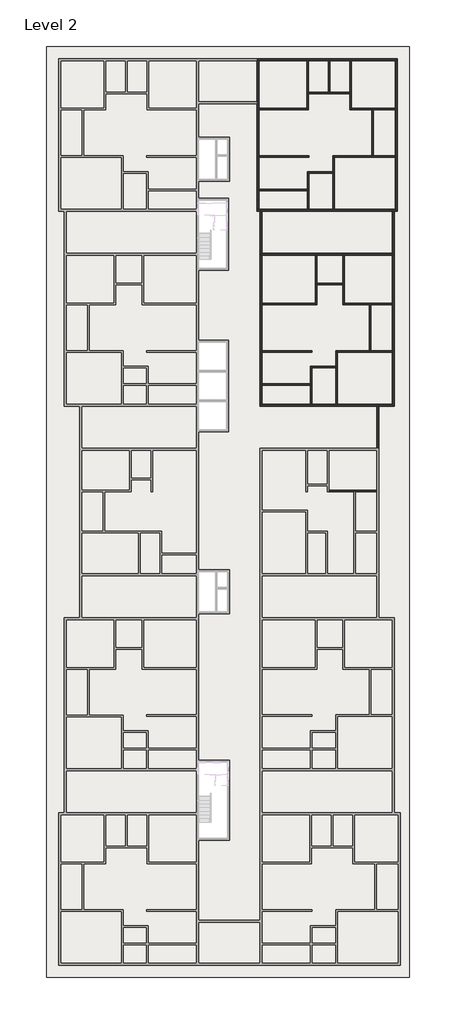
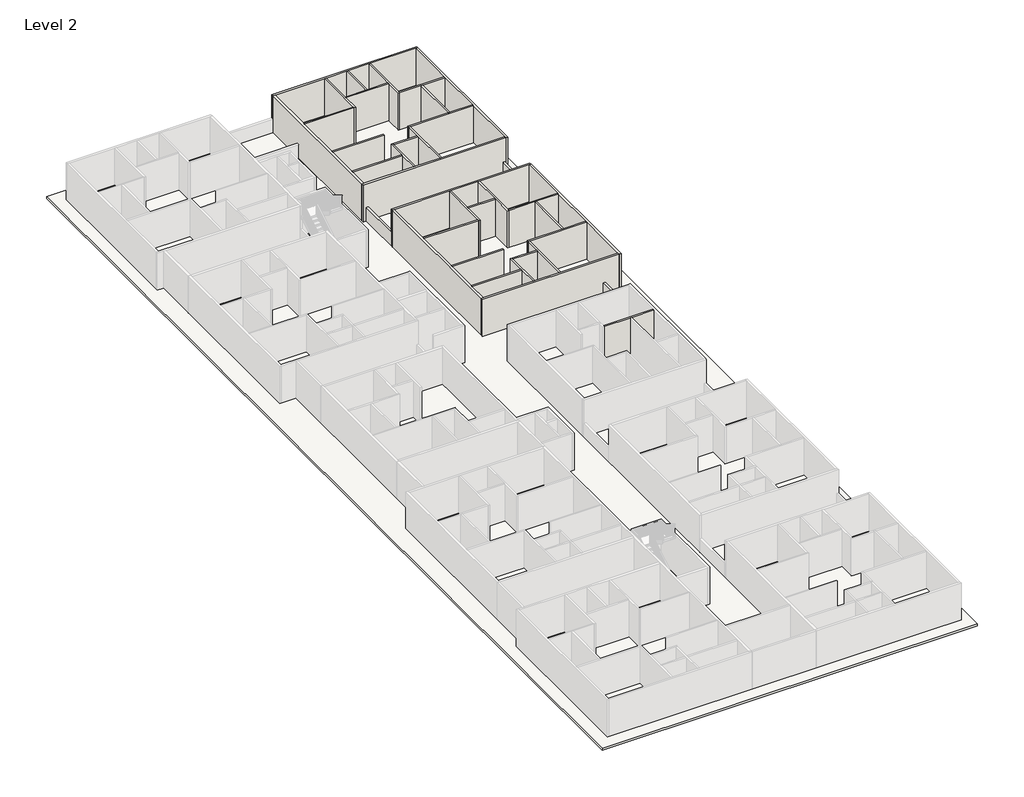
# One storey, part 4 of 8: 37 walls, 1 roof, 1 slab.
"""IFC4 building model written with IfcOpenShell, lengths in millimetres."""

from ifc_helpers import new_model, si_unit, frame, origin, place, context, project, spatial, polyline, outline, extrude, faceted_brep, element, save

model = new_model("IFC4")

# Units and contexts
model_context = context("Model", 3, world=origin())
ifc_project = project(units=[si_unit("LENGTHUNIT", "METRE", prefix="MILLI")], contexts=[model_context])

# Site, building, storey
site = spatial("IfcSite", under=ifc_project)
building = spatial("IfcBuilding", under=site)
storey = spatial("IfcBuildingStorey", under=building, Name="Level 2", Elevation=28282.6172466)

# Roof
placement = place(None, origin())
element("IfcRoof", 1, ObjectType="SLAB", at=placement, inside=storey, context=model_context, shape_type="SweptSolid", body=[
    extrude(outline(polyline([(-15237.9415084, -35021.5344126), (-15237.9415084, 36097.9216096), (12498.9443719, 36097.9216096), (12498.9443719, -35021.5344126), (-15237.9415084, -35021.5344126)]), holes=[polyline([(-3617.4415084, 29152.4900967), (-3617.4415084, 25799.6900967), (-1255.2415084, 25799.6900967), (-1255.2415084, 29152.4900967), (-3617.4415084, 29152.4900967)]), polyline([(-3617.4415084, 24490.1216096), (-3617.4415084, 19003.7216096), (-1331.4415084, 19003.7216096), (-1331.4415084, 24490.1216096), (-3617.4415084, 24490.1216096)]), polyline([(-3617.4415084, 13669.6303368), (-3617.4415084, 6659.2303368), (-1331.4415084, 6659.2303368), (-1331.4415084, 13669.6303368), (-3617.4415084, 13669.6303368)]), polyline([(-3617.4415084, -3882.2751812), (-3617.4415084, -7235.0751812), (-1255.2415084, -7235.0751812), (-1255.2415084, -3882.2751812), (-3617.4415084, -3882.2751812)]), polyline([(-3617.4415084, -18429.9851539), (-3617.4415084, -24525.9851539), (-1229.8415084, -24525.9851539), (-1229.8415084, -18429.9851539), (-3617.4415084, -18429.9851539)])]), frame((0.0, 0.0, 28282.6172466), z_axis=(0.0, 0.0, 1.0), x_axis=(1.0, 0.0, 0.0)), (0.0, 0.0, 1.0), 152.4),
])

# Slab
element("IfcSlab", 2, ObjectType="FLOOR", at=placement, inside=storey, context=model_context, shape_type="SweptSolid", body=[
    extrude(outline(polyline([(-14323.5415084, 35183.5216096), (11584.5443719, 35183.5216096), (11584.5443719, 23499.5216096), (11360.9214687, 23499.5216096), (11360.9214687, 8615.1216096), (10173.4714687, 8615.1216096), (10173.4714687, -7538.7344126), (11360.9214687, -7538.7344126), (11360.9214687, -22423.1344126), (11813.0584916, -22423.1344126), (11813.0584916, -34107.1344126), (11584.5443719, -34107.1344126), (-14323.5415084, -34107.1344126), (-14323.5415084, 35183.5216096)]), holes=[polyline([(-3617.4415084, 29152.4900967), (-3617.4415084, 25799.6900967), (-1255.2415084, 25799.6900967), (-1255.2415084, 29152.4900967), (-3617.4415084, 29152.4900967)]), polyline([(-3617.4415084, 24490.1216096), (-3617.4415084, 19003.7216096), (-1331.4415084, 19003.7216096), (-1331.4415084, 24490.1216096), (-3617.4415084, 24490.1216096)]), polyline([(-3617.4415084, 13669.6303368), (-3617.4415084, 6659.2303368), (-1331.4415084, 6659.2303368), (-1331.4415084, 13669.6303368), (-3617.4415084, 13669.6303368)]), polyline([(-3617.4415084, -3882.2751812), (-3617.4415084, -7235.0751812), (-1255.2415084, -7235.0751812), (-1255.2415084, -3882.2751812), (-3617.4415084, -3882.2751812)]), polyline([(-3617.4415084, -18429.9851539), (-3617.4415084, -24525.9851539), (-1229.8415084, -24525.9851539), (-1229.8415084, -18429.9851539), (-3617.4415084, -18429.9851539)])]), frame((0.0, 0.0, 27673.0172466), z_axis=(0.0, 0.0, 1.0), x_axis=(1.0, 0.0, 0.0)), (0.0, 0.0, 1.0), 609.6),
])

# Walls
element("IfcWall", 3, ObjectType="4.5\"", at=placement, inside=storey, context=model_context, shape_type="Brep", body=[
    faceted_brep([(6363.4714687, 2100.0216096, 28282.6172466), (8282.4584916, 2100.0216096, 28282.6172466), (8396.7584916, 2100.0216096, 28282.6172466), (10021.0714687, 2100.0216096, 28282.6172466), (10021.0714687, 2100.0216096, 31330.6172466), (8396.7584916, 2100.0216096, 31330.6172466), (8282.4584916, 2100.0216096, 31330.6172466), (6363.4714687, 2100.0216096, 31330.6172466), (6363.4714687, 2214.3216096, 28282.6172466), (6363.4714687, 2214.3216096, 31330.6172466), (10021.0714687, 2214.3216096, 31330.6172466), (10021.0714687, 2214.3216096, 28282.6172466)], [[[0, 1, 2, 3, 4, 5, 6, 7]], [[8, 9, 10, 11]], [[3, 2, 1, 0, 8, 11]], [[0, 7, 9, 8]], [[4, 3, 11, 10]], [[7, 6, 5, 4, 10, 9]]]),
])
element("IfcWall", 4, ObjectType="4.5\"", at=placement, inside=storey, context=model_context, shape_type="Brep", body=[
    faceted_brep([(5315.7214687, 20146.7216096, 28282.6172466), (5315.7214687, 16489.1216096, 28282.6172466), (5315.7214687, 16374.8216096, 28282.6172466), (5315.7214687, 16374.8216096, 31330.6172466), (5315.7214687, 16489.1216096, 31330.6172466), (5315.7214687, 20146.7216096, 31330.6172466), (5430.0214687, 20146.7216096, 28282.6172466), (5430.0214687, 20146.7216096, 31330.6172466), (5430.0214687, 18013.1216096, 31330.6172466), (5430.0214687, 17898.8216096, 31330.6172466), (5430.0214687, 16374.8216096, 31330.6172466), (5430.0214687, 16374.8216096, 28282.6172466), (5430.0214687, 17898.8216096, 28282.6172466), (5430.0214687, 18013.1216096, 28282.6172466)], [[[0, 1, 2, 3, 4, 5]], [[6, 7, 8, 9, 10, 11, 12, 13]], [[2, 1, 0, 6, 13, 12, 11]], [[0, 5, 7, 6]], [[3, 2, 11, 10]], [[5, 4, 3, 10, 9, 8, 7]]]),
])
element("IfcWall", 5, ObjectType="4.5\"", at=placement, inside=storey, context=model_context, shape_type="SweptSolid", body=[
    extrude(outline(polyline([(1259.3584916, 16489.1216096), (5315.7214687, 16489.1216096), (5315.7214687, 16374.8216096), (1259.3584916, 16374.8216096), (1259.3584916, 16489.1216096)])), frame((0.0, 0.0, 28282.6172466), z_axis=(0.0, 0.0, 1.0), x_axis=(1.0, 0.0, 0.0)), (0.0, 0.0, 1.0), 3048.0),
])
element("IfcWall", 6, ObjectType="4.5\"", at=placement, inside=storey, context=model_context, shape_type="SweptSolid", body=[
    extrude(outline(polyline([(7436.6214687, 17898.8216096), (5430.0214687, 17898.8216096), (5430.0214687, 18013.1216096), (7436.6214687, 18013.1216096), (7436.6214687, 17898.8216096)])), frame((0.0, 0.0, 28282.6172466), z_axis=(0.0, 0.0, 1.0), x_axis=(1.0, 0.0, 0.0)), (0.0, 0.0, 1.0), 3048.0),
])
element("IfcWall", 7, ObjectType="4.5\"", at=placement, inside=storey, context=model_context, shape_type="Brep", body=[
    faceted_brep([(7436.6214687, 20146.7216096, 28282.6172466), (7436.6214687, 18013.1216096, 28282.6172466), (7436.6214687, 17898.8216096, 28282.6172466), (7436.6214687, 16374.8216096, 28282.6172466), (7436.6214687, 16374.8216096, 31330.6172466), (7436.6214687, 17898.8216096, 31330.6172466), (7436.6214687, 18013.1216096, 31330.6172466), (7436.6214687, 20146.7216096, 31330.6172466), (7550.9214687, 20146.7216096, 28282.6172466), (7550.9214687, 20146.7216096, 31330.6172466), (7550.9214687, 16489.1216096, 31330.6172466), (7550.9214687, 16374.8216096, 31330.6172466), (7550.9214687, 16374.8216096, 28282.6172466), (7550.9214687, 16489.1216096, 28282.6172466)], [[[0, 1, 2, 3, 4, 5, 6, 7]], [[8, 9, 10, 11, 12, 13]], [[3, 2, 1, 0, 8, 13, 12]], [[0, 7, 9, 8]], [[4, 3, 12, 11]], [[7, 6, 5, 4, 11, 10, 9]]]),
])
element("IfcWall", 8, ObjectType="4.5\"", at=placement, inside=storey, context=model_context, shape_type="Brep", body=[
    faceted_brep([(7550.9214687, 16374.8216096, 28282.6172466), (9469.9084916, 16374.8216096, 28282.6172466), (9584.2084916, 16374.8216096, 28282.6172466), (11208.5214687, 16374.8216096, 28282.6172466), (11208.5214687, 16374.8216096, 31330.6172466), (9584.2084916, 16374.8216096, 31330.6172466), (9469.9084916, 16374.8216096, 31330.6172466), (7550.9214687, 16374.8216096, 31330.6172466), (7550.9214687, 16489.1216096, 28282.6172466), (7550.9214687, 16489.1216096, 31330.6172466), (11208.5214687, 16489.1216096, 31330.6172466), (11208.5214687, 16489.1216096, 28282.6172466)], [[[0, 1, 2, 3, 4, 5, 6, 7]], [[8, 9, 10, 11]], [[3, 2, 1, 0, 8, 11]], [[0, 7, 9, 8]], [[4, 3, 11, 10]], [[7, 6, 5, 4, 10, 9]]]),
])
element("IfcWall", 9, ObjectType="4.5\"", at=placement, inside=storey, context=model_context, shape_type="SweptSolid", body=[
    extrude(outline(polyline([(9469.9084916, 12869.6216096), (9469.9084916, 16374.8216096), (9584.2084916, 16374.8216096), (9584.2084916, 12869.6216096), (9469.9084916, 12869.6216096)])), frame((0.0, 0.0, 28282.6172466), z_axis=(0.0, 0.0, 1.0), x_axis=(1.0, 0.0, 0.0)), (0.0, 0.0, 1.0), 3048.0),
])
element("IfcWall", 10, ObjectType="4.5\"", at=placement, inside=storey, context=model_context, shape_type="Brep", body=[
    faceted_brep([(11208.5214687, 12869.6216096, 28282.6172466), (9584.2084916, 12869.6216096, 28282.6172466), (9469.9084916, 12869.6216096, 28282.6172466), (6885.4584916, 12869.6216096, 28282.6172466), (6885.4584916, 12869.6216096, 31330.6172466), (9469.9084916, 12869.6216096, 31330.6172466), (9584.2084916, 12869.6216096, 31330.6172466), (11208.5214687, 12869.6216096, 31330.6172466), (11208.5214687, 12755.3216096, 28282.6172466), (11208.5214687, 12755.3216096, 31330.6172466), (6999.7584916, 12755.3216096, 31330.6172466), (6885.4584916, 12755.3216096, 31330.6172466), (6885.4584916, 12755.3216096, 28282.6172466), (6999.7584916, 12755.3216096, 28282.6172466)], [[[0, 1, 2, 3, 4, 5, 6, 7]], [[8, 9, 10, 11, 12, 13]], [[3, 2, 1, 0, 8, 13, 12]], [[0, 7, 9, 8]], [[4, 3, 12, 11]], [[7, 6, 5, 4, 11, 10, 9]]]),
])
element("IfcWall", 11, ObjectType="4.5\"", at=placement, inside=storey, context=model_context, shape_type="Brep", body=[
    faceted_brep([(6885.4584916, 12755.3216096, 28282.6172466), (6885.4584916, 11663.1216096, 28282.6172466), (6885.4584916, 11548.8216096, 28282.6172466), (6885.4584916, 8767.5216096, 28282.6172466), (6885.4584916, 8767.5216096, 31330.6172466), (6885.4584916, 11548.8216096, 31330.6172466), (6885.4584916, 11663.1216096, 31330.6172466), (6885.4584916, 12755.3216096, 31330.6172466), (6999.7584916, 12755.3216096, 28282.6172466), (6999.7584916, 12755.3216096, 31330.6172466), (6999.7584916, 8767.5216096, 31330.6172466), (6999.7584916, 8767.5216096, 28282.6172466)], [[[0, 1, 2, 3, 4, 5, 6, 7]], [[8, 9, 10, 11]], [[3, 2, 1, 0, 8, 11]], [[0, 7, 9, 8]], [[4, 3, 11, 10]], [[7, 6, 5, 4, 10, 9]]]),
])
element("IfcWall", 12, ObjectType="4.5\"", at=placement, inside=storey, context=model_context, shape_type="Brep", body=[
    faceted_brep([(5056.6584916, 8767.5216096, 28282.6172466), (5056.6584916, 11548.8216096, 28282.6172466), (5056.6584916, 11663.1216096, 28282.6172466), (5056.6584916, 11663.1216096, 31330.6172466), (5056.6584916, 11548.8216096, 31330.6172466), (5056.6584916, 8767.5216096, 31330.6172466), (4942.3584916, 8767.5216096, 28282.6172466), (4942.3584916, 8767.5216096, 31330.6172466), (4942.3584916, 10215.3216096, 31330.6172466), (4942.3584916, 10329.6216096, 31330.6172466), (4942.3584916, 11663.1216096, 31330.6172466), (4942.3584916, 11663.1216096, 28282.6172466), (4942.3584916, 10329.6216096, 28282.6172466), (4942.3584916, 10215.3216096, 28282.6172466)], [[[0, 1, 2, 3, 4, 5]], [[6, 7, 8, 9, 10, 11, 12, 13]], [[2, 1, 0, 6, 13, 12, 11]], [[0, 5, 7, 6]], [[3, 2, 11, 10]], [[5, 4, 3, 10, 9, 8, 7]]]),
])
element("IfcWall", 13, ObjectType="4.5\"", at=placement, inside=storey, context=model_context, shape_type="SweptSolid", body=[
    extrude(outline(polyline([(6885.4584916, 11548.8216096), (5056.6584916, 11548.8216096), (5056.6584916, 11663.1216096), (6885.4584916, 11663.1216096), (6885.4584916, 11548.8216096)])), frame((0.0, 0.0, 28282.6172466), z_axis=(0.0, 0.0, 1.0), x_axis=(1.0, 0.0, 0.0)), (0.0, 0.0, 1.0), 3048.0),
])
element("IfcWall", 14, ObjectType="4.5\"", at=placement, inside=storey, context=model_context, shape_type="SweptSolid", body=[
    extrude(outline(polyline([(4942.3584916, 10215.3216096), (1259.3584916, 10215.3216096), (1259.3584916, 10329.6216096), (4942.3584916, 10329.6216096), (4942.3584916, 10215.3216096)])), frame((0.0, 0.0, 28282.6172466), z_axis=(0.0, 0.0, 1.0), x_axis=(1.0, 0.0, 0.0)), (0.0, 0.0, 1.0), 3048.0),
])
element("IfcWall", 15, ObjectType="4.5\"", at=placement, inside=storey, context=model_context, shape_type="SweptSolid", body=[
    extrude(outline(polyline([(5056.6584916, 12755.3216096), (1259.3584916, 12755.3216096), (1259.3584916, 12869.6216096), (5056.6584916, 12869.6216096), (5056.6584916, 12755.3216096)])), frame((0.0, 0.0, 28282.6172466), z_axis=(0.0, 0.0, 1.0), x_axis=(1.0, 0.0, 0.0)), (0.0, 0.0, 1.0), 3048.0),
])
element("IfcWall", 16, ObjectType="4.5\"", at=placement, inside=storey, context=model_context, shape_type="Brep", body=[
    faceted_brep([(4688.4443719, 35031.1216096, 28282.6172466), (4688.4443719, 31373.5216096, 28282.6172466), (4688.4443719, 31259.2216096, 28282.6172466), (4688.4443719, 31259.2216096, 31330.6172466), (4688.4443719, 31373.5216096, 31330.6172466), (4688.4443719, 35031.1216096, 31330.6172466), (4802.7443719, 35031.1216096, 28282.6172466), (4802.7443719, 35031.1216096, 31330.6172466), (4802.7443719, 32592.7216096, 31330.6172466), (4802.7443719, 32478.4216096, 31330.6172466), (4802.7443719, 31259.2216096, 31330.6172466), (4802.7443719, 31259.2216096, 28282.6172466), (4802.7443719, 32478.4216096, 28282.6172466), (4802.7443719, 32592.7216096, 28282.6172466)], [[[0, 1, 2, 3, 4, 5]], [[6, 7, 8, 9, 10, 11, 12, 13]], [[2, 1, 0, 6, 13, 12, 11]], [[0, 5, 7, 6]], [[3, 2, 11, 10]], [[5, 4, 3, 10, 9, 8, 7]]]),
])
element("IfcWall", 17, ObjectType="4.5\"", at=placement, inside=storey, context=model_context, shape_type="SweptSolid", body=[
    extrude(outline(polyline([(1030.8443719, 31373.5216096), (4688.4443719, 31373.5216096), (4688.4443719, 31259.2216096), (1030.8443719, 31259.2216096), (1030.8443719, 31373.5216096)])), frame((0.0, 0.0, 28282.6172466), z_axis=(0.0, 0.0, 1.0), x_axis=(1.0, 0.0, 0.0)), (0.0, 0.0, 1.0), 3048.0),
])
element("IfcWall", 18, ObjectType="4.5\"", at=placement, inside=storey, context=model_context, shape_type="Brep", body=[
    faceted_brep([(4802.7443719, 32478.4216096, 28282.6172466), (7965.0443719, 32478.4216096, 28282.6172466), (7965.0443719, 32478.4216096, 31330.6172466), (4802.7443719, 32478.4216096, 31330.6172466), (4802.7443719, 32592.7216096, 28282.6172466), (4802.7443719, 32592.7216096, 31330.6172466), (6326.7443719, 32592.7216096, 31330.6172466), (6441.0443719, 32592.7216096, 31330.6172466), (7965.0443719, 32592.7216096, 31330.6172466), (7965.0443719, 32592.7216096, 28282.6172466), (6441.0443719, 32592.7216096, 28282.6172466), (6326.7443719, 32592.7216096, 28282.6172466)], [[[0, 1, 2, 3]], [[4, 5, 6, 7, 8, 9, 10, 11]], [[1, 0, 4, 11, 10, 9]], [[0, 3, 5, 4]], [[2, 1, 9, 8]], [[3, 2, 8, 7, 6, 5]]]),
])
element("IfcWall", 19, ObjectType="4.5\"", at=placement, inside=storey, context=model_context, shape_type="SweptSolid", body=[
    extrude(outline(polyline([(6326.7443719, 32592.7216096), (6326.7443719, 35031.1216096), (6441.0443719, 35031.1216096), (6441.0443719, 32592.7216096), (6326.7443719, 32592.7216096)])), frame((0.0, 0.0, 28282.6172466), z_axis=(0.0, 0.0, 1.0), x_axis=(1.0, 0.0, 0.0)), (0.0, 0.0, 1.0), 3048.0),
])
element("IfcWall", 20, ObjectType="4.5\"", at=placement, inside=storey, context=model_context, shape_type="Brep", body=[
    faceted_brep([(7965.0443719, 35031.1216096, 28282.6172466), (7965.0443719, 32592.7216096, 28282.6172466), (7965.0443719, 32478.4216096, 28282.6172466), (7965.0443719, 31259.2216096, 28282.6172466), (7965.0443719, 31259.2216096, 31330.6172466), (7965.0443719, 32478.4216096, 31330.6172466), (7965.0443719, 32592.7216096, 31330.6172466), (7965.0443719, 35031.1216096, 31330.6172466), (8079.3443719, 35031.1216096, 28282.6172466), (8079.3443719, 35031.1216096, 31330.6172466), (8079.3443719, 31373.5216096, 31330.6172466), (8079.3443719, 31259.2216096, 31330.6172466), (8079.3443719, 31259.2216096, 28282.6172466), (8079.3443719, 31373.5216096, 28282.6172466)], [[[0, 1, 2, 3, 4, 5, 6, 7]], [[8, 9, 10, 11, 12, 13]], [[3, 2, 1, 0, 8, 13, 12]], [[0, 7, 9, 8]], [[4, 3, 12, 11]], [[7, 6, 5, 4, 11, 10, 9]]]),
])
element("IfcWall", 21, ObjectType="4.5\"", at=placement, inside=storey, context=model_context, shape_type="Brep", body=[
    faceted_brep([(8079.3443719, 31259.2216096, 28282.6172466), (9641.4443719, 31259.2216096, 28282.6172466), (9755.7443719, 31259.2216096, 28282.6172466), (11432.1443719, 31259.2216096, 28282.6172466), (11432.1443719, 31259.2216096, 31330.6172466), (9755.7443719, 31259.2216096, 31330.6172466), (9641.4443719, 31259.2216096, 31330.6172466), (8079.3443719, 31259.2216096, 31330.6172466), (8079.3443719, 31373.5216096, 28282.6172466), (8079.3443719, 31373.5216096, 31330.6172466), (11432.1443719, 31373.5216096, 31330.6172466), (11432.1443719, 31373.5216096, 28282.6172466)], [[[0, 1, 2, 3, 4, 5, 6, 7]], [[8, 9, 10, 11]], [[3, 2, 1, 0, 8, 11]], [[0, 7, 9, 8]], [[4, 3, 11, 10]], [[7, 6, 5, 4, 10, 9]]]),
])
element("IfcWall", 22, ObjectType="4.5\"", at=placement, inside=storey, context=model_context, shape_type="SweptSolid", body=[
    extrude(outline(polyline([(9641.4443719, 27754.0216096), (9641.4443719, 31259.2216096), (9755.7443719, 31259.2216096), (9755.7443719, 27754.0216096), (9641.4443719, 27754.0216096)])), frame((0.0, 0.0, 28282.6172466), z_axis=(0.0, 0.0, 1.0), x_axis=(1.0, 0.0, 0.0)), (0.0, 0.0, 1.0), 3048.0),
])
element("IfcWall", 23, ObjectType="4.5\"", at=placement, inside=storey, context=model_context, shape_type="Brep", body=[
    faceted_brep([(11432.1443719, 27754.0216096, 28282.6172466), (9755.7443719, 27754.0216096, 28282.6172466), (9641.4443719, 27754.0216096, 28282.6172466), (6656.9443719, 27754.0216096, 28282.6172466), (6656.9443719, 27754.0216096, 31330.6172466), (9641.4443719, 27754.0216096, 31330.6172466), (9755.7443719, 27754.0216096, 31330.6172466), (11432.1443719, 27754.0216096, 31330.6172466), (11432.1443719, 27639.7216096, 28282.6172466), (11432.1443719, 27639.7216096, 31330.6172466), (6771.2443719, 27639.7216096, 31330.6172466), (6656.9443719, 27639.7216096, 31330.6172466), (6656.9443719, 27639.7216096, 28282.6172466), (6771.2443719, 27639.7216096, 28282.6172466)], [[[0, 1, 2, 3, 4, 5, 6, 7]], [[8, 9, 10, 11, 12, 13]], [[3, 2, 1, 0, 8, 13, 12]], [[0, 7, 9, 8]], [[4, 3, 12, 11]], [[7, 6, 5, 4, 11, 10, 9]]]),
])
element("IfcWall", 24, ObjectType="4.5\"", at=placement, inside=storey, context=model_context, shape_type="Brep", body=[
    faceted_brep([(6656.9443719, 27639.7216096, 28282.6172466), (6656.9443719, 26547.5216096, 28282.6172466), (6656.9443719, 26433.2216096, 28282.6172466), (6656.9443719, 23651.9216096, 28282.6172466), (6656.9443719, 23651.9216096, 31330.6172466), (6656.9443719, 26433.2216096, 31330.6172466), (6656.9443719, 26547.5216096, 31330.6172466), (6656.9443719, 27639.7216096, 31330.6172466), (6771.2443719, 27639.7216096, 28282.6172466), (6771.2443719, 27639.7216096, 31330.6172466), (6771.2443719, 23651.9216096, 31330.6172466), (6771.2443719, 23651.9216096, 28282.6172466)], [[[0, 1, 2, 3, 4, 5, 6, 7]], [[8, 9, 10, 11]], [[3, 2, 1, 0, 8, 11]], [[0, 7, 9, 8]], [[4, 3, 11, 10]], [[7, 6, 5, 4, 10, 9]]]),
])
element("IfcWall", 25, ObjectType="4.5\"", at=placement, inside=storey, context=model_context, shape_type="SweptSolid", body=[
    extrude(outline(polyline([(4713.8443719, 25099.7216096), (1030.8443719, 25099.7216096), (1030.8443719, 25214.0216096), (4713.8443719, 25214.0216096), (4713.8443719, 25099.7216096)])), frame((0.0, 0.0, 28282.6172466), z_axis=(0.0, 0.0, 1.0), x_axis=(1.0, 0.0, 0.0)), (0.0, 0.0, 1.0), 3048.0),
])
element("IfcWall", 26, ObjectType="4.5\"", at=placement, inside=storey, context=model_context, shape_type="Brep", body=[
    faceted_brep([(4828.1443719, 23651.9216096, 28282.6172466), (4828.1443719, 26433.2216096, 28282.6172466), (4828.1443719, 26547.5216096, 28282.6172466), (4828.1443719, 26547.5216096, 31330.6172466), (4828.1443719, 26433.2216096, 31330.6172466), (4828.1443719, 23651.9216096, 31330.6172466), (4713.8443719, 23651.9216096, 28282.6172466), (4713.8443719, 23651.9216096, 31330.6172466), (4713.8443719, 25099.7216096, 31330.6172466), (4713.8443719, 25214.0216096, 31330.6172466), (4713.8443719, 26547.5216096, 31330.6172466), (4713.8443719, 26547.5216096, 28282.6172466), (4713.8443719, 25214.0216096, 28282.6172466), (4713.8443719, 25099.7216096, 28282.6172466)], [[[0, 1, 2, 3, 4, 5]], [[6, 7, 8, 9, 10, 11, 12, 13]], [[2, 1, 0, 6, 13, 12, 11]], [[0, 5, 7, 6]], [[3, 2, 11, 10]], [[5, 4, 3, 10, 9, 8, 7]]]),
])
element("IfcWall", 27, ObjectType="4.5\"", at=placement, inside=storey, context=model_context, shape_type="SweptSolid", body=[
    extrude(outline(polyline([(6656.9443719, 26433.2216096), (4828.1443719, 26433.2216096), (4828.1443719, 26547.5216096), (6656.9443719, 26547.5216096), (6656.9443719, 26433.2216096)])), frame((0.0, 0.0, 28282.6172466), z_axis=(0.0, 0.0, 1.0), x_axis=(1.0, 0.0, 0.0)), (0.0, 0.0, 1.0), 3048.0),
])
element("IfcWall", 28, ObjectType="4.5\"", at=placement, inside=storey, context=model_context, shape_type="SweptSolid", body=[
    extrude(outline(polyline([(4828.1443719, 27639.7216096), (1030.8443719, 27639.7216096), (1030.8443719, 27754.0216096), (4828.1443719, 27754.0216096), (4828.1443719, 27639.7216096)])), frame((0.0, 0.0, 28282.6172466), z_axis=(0.0, 0.0, 1.0), x_axis=(1.0, 0.0, 0.0)), (0.0, 0.0, 1.0), 3048.0),
])
element("IfcWall", 29, ObjectType="6\"", at=placement, inside=storey, context=model_context, shape_type="Brep", body=[
    faceted_brep([(1106.9584916, 20146.7216096, 31330.6172466), (1106.9584916, 20146.7216096, 28282.6172466), (1259.3584916, 20146.7216096, 28282.6172466), (5315.7214687, 20146.7216096, 28282.6172466), (5430.0214687, 20146.7216096, 28282.6172466), (7436.6214687, 20146.7216096, 28282.6172466), (7550.9214687, 20146.7216096, 28282.6172466), (11208.5214687, 20146.7216096, 28282.6172466), (11360.9214687, 20146.7216096, 28282.6172466), (11360.9214687, 20146.7216096, 31330.6172466), (11208.5214687, 20146.7216096, 31330.6172466), (7550.9214687, 20146.7216096, 31330.6172466), (7436.6214687, 20146.7216096, 31330.6172466), (5430.0214687, 20146.7216096, 31330.6172466), (5315.7214687, 20146.7216096, 31330.6172466), (1259.3584916, 20146.7216096, 31330.6172466), (1106.9584916, 20299.1216096, 28282.6172466), (1106.9584916, 20299.1216096, 29501.8172466), (1106.9584916, 20299.1216096, 31330.6172466), (11360.9214687, 20299.1216096, 31330.6172466), (11360.9214687, 20299.1216096, 29501.8172466), (11360.9214687, 20299.1216096, 28282.6172466), (11208.5214687, 20299.1216096, 28282.6172466), (1259.3584916, 20299.1216096, 28282.6172466)], [[[0, 1, 2, 3, 4, 5, 6, 7, 8, 9, 10, 11, 12, 13, 14, 15]], [[16, 17, 18, 19, 20, 21, 22, 23]], [[8, 7, 6, 5, 4, 3, 2, 1, 16, 23, 22, 21]], [[0, 18, 17, 16, 1]], [[8, 21, 20, 19, 9]], [[0, 15, 14, 13, 12, 11, 10, 9, 19, 18]]]),
])
element("IfcWall", 30, ObjectType="6\"", at=placement, inside=storey, context=model_context, shape_type="Brep", body=[
    faceted_brep([(11208.5214687, 20146.7216096, 31330.6172466), (11208.5214687, 20146.7216096, 28282.6172466), (11208.5214687, 16489.1216096, 28282.6172466), (11208.5214687, 16374.8216096, 28282.6172466), (11208.5214687, 12869.6216096, 28282.6172466), (11208.5214687, 12755.3216096, 28282.6172466), (11208.5214687, 8767.5216096, 28282.6172466), (11208.5214687, 8615.1216096, 28282.6172466), (11208.5214687, 8615.1216096, 31330.6172466), (11208.5214687, 8767.5216096, 31330.6172466), (11208.5214687, 12755.3216096, 31330.6172466), (11208.5214687, 12869.6216096, 31330.6172466), (11208.5214687, 16374.8216096, 31330.6172466), (11208.5214687, 16489.1216096, 31330.6172466), (11360.9214687, 20146.7216096, 28282.6172466), (11360.9214687, 20146.7216096, 31330.6172466), (11360.9214687, 8615.1216096, 31330.6172466), (11360.9214687, 8615.1216096, 28282.6172466)], [[[0, 1, 2, 3, 4, 5, 6, 7, 8, 9, 10, 11, 12, 13]], [[14, 15, 16, 17]], [[7, 6, 5, 4, 3, 2, 1, 14, 17]], [[8, 7, 17, 16]], [[0, 15, 14, 1]], [[0, 13, 12, 11, 10, 9, 8, 16, 15]]]),
])
element("IfcWall", 31, ObjectType="6\"", at=placement, inside=storey, context=model_context, shape_type="Brep", body=[
    faceted_brep([(11208.5214687, 8767.5216096, 28282.6172466), (6999.7584916, 8767.5216096, 28282.6172466), (6885.4584916, 8767.5216096, 28282.6172466), (5056.6584916, 8767.5216096, 28282.6172466), (4942.3584916, 8767.5216096, 28282.6172466), (1259.3584916, 8767.5216096, 28282.6172466), (1106.9584916, 8767.5216096, 28282.6172466), (1106.9584916, 8767.5216096, 31330.6172466), (1259.3584916, 8767.5216096, 31330.6172466), (4942.3584916, 8767.5216096, 31330.6172466), (5056.6584916, 8767.5216096, 31330.6172466), (6885.4584916, 8767.5216096, 31330.6172466), (6999.7584916, 8767.5216096, 31330.6172466), (11208.5214687, 8767.5216096, 31330.6172466), (11208.5214687, 8615.1216096, 28282.6172466), (11208.5214687, 8615.1216096, 31330.6172466), (1106.9584916, 8615.1216096, 31330.6172466), (1106.9584916, 8615.1216096, 28282.6172466), (10021.0714687, 8615.1216096, 28282.6172466), (10173.4714687, 8615.1216096, 28282.6172466)], [[[0, 1, 2, 3, 4, 5, 6, 7, 8, 9, 10, 11, 12, 13]], [[14, 15, 16, 17, 18, 19]], [[6, 5, 4, 3, 2, 1, 0, 14, 19, 18, 17]], [[0, 13, 15, 14]], [[7, 6, 17, 16]], [[13, 12, 11, 10, 9, 8, 7, 16, 15]]]),
])
element("IfcWall", 32, ObjectType="6\"", at=placement, inside=storey, context=model_context, shape_type="Brep", body=[
    faceted_brep([(1259.3584916, 8767.5216096, 28282.6172466), (1259.3584916, 10215.3216096, 28282.6172466), (1259.3584916, 10329.6216096, 28282.6172466), (1259.3584916, 12755.3216096, 28282.6172466), (1259.3584916, 12869.6216096, 28282.6172466), (1259.3584916, 16374.8216096, 28282.6172466), (1259.3584916, 16489.1216096, 28282.6172466), (1259.3584916, 20146.7216096, 28282.6172466), (1259.3584916, 20146.7216096, 31330.6172466), (1259.3584916, 16489.1216096, 31330.6172466), (1259.3584916, 16374.8216096, 31330.6172466), (1259.3584916, 12869.6216096, 31330.6172466), (1259.3584916, 12755.3216096, 31330.6172466), (1259.3584916, 10329.6216096, 31330.6172466), (1259.3584916, 10215.3216096, 31330.6172466), (1259.3584916, 8767.5216096, 31330.6172466), (1106.9584916, 8767.5216096, 28282.6172466), (1106.9584916, 8767.5216096, 31330.6172466), (1106.9584916, 20146.7216096, 31330.6172466), (1106.9584916, 20146.7216096, 28282.6172466)], [[[0, 1, 2, 3, 4, 5, 6, 7, 8, 9, 10, 11, 12, 13, 14, 15]], [[16, 17, 18, 19]], [[7, 6, 5, 4, 3, 2, 1, 0, 16, 19]], [[0, 15, 17, 16]], [[7, 19, 18, 8]], [[15, 14, 13, 12, 11, 10, 9, 8, 18, 17]]]),
])
element("IfcWall", 33, ObjectType="6\"", at=placement, inside=storey, context=model_context, shape_type="Brep", body=[
    faceted_brep([(878.4443719, 35031.1216096, 31330.6172466), (878.4443719, 35031.1216096, 28282.6172466), (1030.8443719, 35031.1216096, 28282.6172466), (4688.4443719, 35031.1216096, 28282.6172466), (4802.7443719, 35031.1216096, 28282.6172466), (6326.7443719, 35031.1216096, 28282.6172466), (6441.0443719, 35031.1216096, 28282.6172466), (7965.0443719, 35031.1216096, 28282.6172466), (8079.3443719, 35031.1216096, 28282.6172466), (11432.1443719, 35031.1216096, 28282.6172466), (11584.5443719, 35031.1216096, 28282.6172466), (11584.5443719, 35031.1216096, 31330.6172466), (11432.1443719, 35031.1216096, 31330.6172466), (8079.3443719, 35031.1216096, 31330.6172466), (7965.0443719, 35031.1216096, 31330.6172466), (6441.0443719, 35031.1216096, 31330.6172466), (6326.7443719, 35031.1216096, 31330.6172466), (4802.7443719, 35031.1216096, 31330.6172466), (4688.4443719, 35031.1216096, 31330.6172466), (1030.8443719, 35031.1216096, 31330.6172466), (878.4443719, 35183.5216096, 28282.6172466), (878.4443719, 35183.5216096, 31330.6172466), (11584.5443719, 35183.5216096, 31330.6172466), (11584.5443719, 35183.5216096, 28282.6172466)], [[[0, 1, 2, 3, 4, 5, 6, 7, 8, 9, 10, 11, 12, 13, 14, 15, 16, 17, 18, 19]], [[20, 21, 22, 23]], [[10, 9, 8, 7, 6, 5, 4, 3, 2, 1, 20, 23]], [[11, 10, 23, 22]], [[0, 21, 20, 1]], [[0, 19, 18, 17, 16, 15, 14, 13, 12, 11, 22, 21]]]),
])
element("IfcWall", 34, ObjectType="6\"", at=placement, inside=storey, context=model_context, shape_type="Brep", body=[
    faceted_brep([(11432.1443719, 35031.1216096, 28282.6172466), (11432.1443719, 31373.5216096, 28282.6172466), (11432.1443719, 31259.2216096, 28282.6172466), (11432.1443719, 27754.0216096, 28282.6172466), (11432.1443719, 27639.7216096, 28282.6172466), (11432.1443719, 23651.9216096, 28282.6172466), (11432.1443719, 23499.5216096, 28282.6172466), (11432.1443719, 23499.5216096, 31330.6172466), (11432.1443719, 23651.9216096, 31330.6172466), (11432.1443719, 27639.7216096, 31330.6172466), (11432.1443719, 27754.0216096, 31330.6172466), (11432.1443719, 31259.2216096, 31330.6172466), (11432.1443719, 31373.5216096, 31330.6172466), (11432.1443719, 35031.1216096, 31330.6172466), (11584.5443719, 35031.1216096, 28282.6172466), (11584.5443719, 35031.1216096, 31330.6172466), (11584.5443719, 23499.5216096, 31330.6172466), (11584.5443719, 23499.5216096, 28282.6172466)], [[[0, 1, 2, 3, 4, 5, 6, 7, 8, 9, 10, 11, 12, 13]], [[14, 15, 16, 17]], [[6, 5, 4, 3, 2, 1, 0, 14, 17]], [[0, 13, 15, 14]], [[7, 6, 17, 16]], [[13, 12, 11, 10, 9, 8, 7, 16, 15]]]),
])
element("IfcWall", 35, ObjectType="6\"", at=placement, inside=storey, context=model_context, shape_type="Brep", body=[
    faceted_brep([(11432.1443719, 23651.9216096, 28282.6172466), (6771.2443719, 23651.9216096, 28282.6172466), (6656.9443719, 23651.9216096, 28282.6172466), (4828.1443719, 23651.9216096, 28282.6172466), (4713.8443719, 23651.9216096, 28282.6172466), (1030.8443719, 23651.9216096, 28282.6172466), (878.4443719, 23651.9216096, 28282.6172466), (878.4443719, 23651.9216096, 31330.6172466), (1030.8443719, 23651.9216096, 31330.6172466), (4713.8443719, 23651.9216096, 31330.6172466), (4828.1443719, 23651.9216096, 31330.6172466), (6656.9443719, 23651.9216096, 31330.6172466), (6771.2443719, 23651.9216096, 31330.6172466), (11432.1443719, 23651.9216096, 31330.6172466), (11432.1443719, 23499.5216096, 28282.6172466), (11432.1443719, 23499.5216096, 31330.6172466), (878.4443719, 23499.5216096, 31330.6172466), (878.4443719, 23499.5216096, 28282.6172466), (1106.9584916, 23499.5216096, 28282.6172466), (1259.3584916, 23499.5216096, 28282.6172466), (11208.5214687, 23499.5216096, 28282.6172466), (11360.9214687, 23499.5216096, 28282.6172466)], [[[0, 1, 2, 3, 4, 5, 6, 7, 8, 9, 10, 11, 12, 13]], [[14, 15, 16, 17, 18, 19, 20, 21]], [[6, 5, 4, 3, 2, 1, 0, 14, 21, 20, 19, 18, 17]], [[0, 13, 15, 14]], [[7, 6, 17, 16]], [[13, 12, 11, 10, 9, 8, 7, 16, 15]]]),
])
element("IfcWall", 36, ObjectType="6\"", at=placement, inside=storey, context=model_context, shape_type="Brep", body=[
    faceted_brep([(1030.8443719, 23651.9216096, 28282.6172466), (1030.8443719, 25099.7216096, 28282.6172466), (1030.8443719, 25214.0216096, 28282.6172466), (1030.8443719, 27639.7216096, 28282.6172466), (1030.8443719, 27754.0216096, 28282.6172466), (1030.8443719, 31259.2216096, 28282.6172466), (1030.8443719, 31373.5216096, 28282.6172466), (1030.8443719, 35031.1216096, 28282.6172466), (1030.8443719, 35031.1216096, 31330.6172466), (1030.8443719, 31373.5216096, 31330.6172466), (1030.8443719, 31259.2216096, 31330.6172466), (1030.8443719, 27754.0216096, 31330.6172466), (1030.8443719, 27639.7216096, 31330.6172466), (1030.8443719, 25214.0216096, 31330.6172466), (1030.8443719, 25099.7216096, 31330.6172466), (1030.8443719, 23651.9216096, 31330.6172466), (878.4443719, 23651.9216096, 28282.6172466), (878.4443719, 23651.9216096, 31330.6172466), (878.4443719, 35031.1216096, 31330.6172466), (878.4443719, 35031.1216096, 28282.6172466), (878.4443719, 31897.3197155, 28282.6172466), (878.4443719, 31744.9197155, 28282.6172466)], [[[0, 1, 2, 3, 4, 5, 6, 7, 8, 9, 10, 11, 12, 13, 14, 15]], [[16, 17, 18, 19, 20, 21]], [[7, 6, 5, 4, 3, 2, 1, 0, 16, 21, 20, 19]], [[0, 15, 17, 16]], [[7, 19, 18, 8]], [[15, 14, 13, 12, 11, 10, 9, 8, 18, 17]]]),
])
element("IfcWall", 37, ObjectType="6\" 2", at=placement, inside=storey, context=model_context, shape_type="SweptSolid", body=[
    extrude(outline(polyline([(1106.9584916, 20299.1216096), (1106.9584916, 23499.5216096), (1259.3584916, 23499.5216096), (1259.3584916, 20299.1216096), (1106.9584916, 20299.1216096)])), frame((0.0, 0.0, 28282.6172466), z_axis=(0.0, 0.0, 1.0), x_axis=(1.0, 0.0, 0.0)), (0.0, 0.0, 1.0), 1219.2),
])
element("IfcWall", 38, ObjectType="6\" 2", at=placement, inside=storey, context=model_context, shape_type="SweptSolid", body=[
    extrude(outline(polyline([(11208.5214687, 20299.1216096), (11208.5214687, 23499.5216096), (11360.9214687, 23499.5216096), (11360.9214687, 20299.1216096), (11208.5214687, 20299.1216096)])), frame((0.0, 0.0, 28282.6172466), z_axis=(0.0, 0.0, 1.0), x_axis=(1.0, 0.0, 0.0)), (0.0, 0.0, 1.0), 1219.2),
])
element("IfcWall", 39, ObjectType="6\" 2", at=placement, inside=storey, context=model_context, shape_type="SweptSolid", body=[
    extrude(outline(polyline([(10021.0714687, 5414.7216096), (10021.0714687, 8615.1216096), (10173.4714687, 8615.1216096), (10173.4714687, 5414.7216096), (10021.0714687, 5414.7216096)])), frame((0.0, 0.0, 28282.6172466), z_axis=(0.0, 0.0, 1.0), x_axis=(1.0, 0.0, 0.0)), (0.0, 0.0, 1.0), 1219.2),
])

save(model, "model.ifc")

# Revit data of these elements
# Type "SLAB"
#   Assembly Code = "B1020"
#   Layers, outside or top first: 0' - 6" "Damp-proofing" (function 1)
# Type "FLOOR"
#   Assembly Code = "B1010"
#   Function = 0
#   Layers, outside or top first: 2' - 0" "Tile, Porcelain, 4in" (function 1)
# Type "4.5\""
#   Assembly Code = "B2010"
#   Layers, outside or top first: 0' - 4 1/2" "WALLS" (function 1)
# Type "6\""
#   Assembly Code = "B2010"
#   Layers, outside or top first: 0' - 6" "WALLS" (function 1)
# Type "6\" 2"
#   Assembly Code = "B2010"
#   Layers, outside or top first: 0' - 6" "4'" (function 1)
# Element 1 (IfcRoof, "SLAB")
#   built-in parameter 1001705 = 93.2907 (stored number, unit not read)
#   built-in parameter 1001710 = 33615
#   Phase Created = New Construction
#   Materials on its faces: "Damp-proofing"
# Element 2 (IfcSlab, "FLOOR")
#   built-in parameter 1001955 = 3.14159 (stored number, unit not read)
#   Height Offset From Level = 0' - 0"
#   Phase Created = New Construction
#   Materials on its faces: "Tile, Porcelain, 4in"
# Elements 3, 4, 5, 6, 7, 8, 9, 10, 11, 12, 13, 14, 15, 16, 17, 18, 19, 20, 21, 22, 23, 24, 25, 26, 27, 28 (IfcWall, "4.5\"")
#   Top Offset = 0' - 0"
#   Base Offset = 0' - 0"
#   Unconnected Height = 10' - 0"
#   wall height = 10' - 0"
#   Phase Created = New Construction
#   Base Constraint = Level 2
#   Materials on its faces: "WALLS"
# Elements 29, 30, 31, 32, 33, 34, 35, 36 (IfcWall, "6\"")
#   Top Offset = 0' - 0"
#   Base Offset = 0' - 0"
#   Unconnected Height = 10' - 0"
#   wall height = 10' - 0"
#   Phase Created = New Construction
#   Base Constraint = Level 2
#   Materials on its faces: "WALLS"
# Elements 37, 38, 39 (IfcWall, "6\" 2")
#   Top Offset = 0' - 0"
#   Base Offset = 0' - 0"
#   Unconnected Height = 4' - 0"
#   wall height = 4' - 0"
#   Phase Created = New Construction
#   Base Constraint = Level 2
#   Materials on its faces: "4'"
# Materials
#   "Damp-proofing": class "Generic", colour RGB 127 127 127, transparency 0, Description = "Damp-proofing", Cost = 0
#   "Tile, Porcelain, 4in": class "Generic", colour RGB 89 87 158, transparency 0, Description = "Porcelain tile, 4\", white", Cost = 0
#   "WALLS": class "Generic", colour RGB 120 120 120, transparency 0, Cost = 0
#   "4'": class "Generic", colour RGB 120 120 120, transparency 0, Cost = 0
